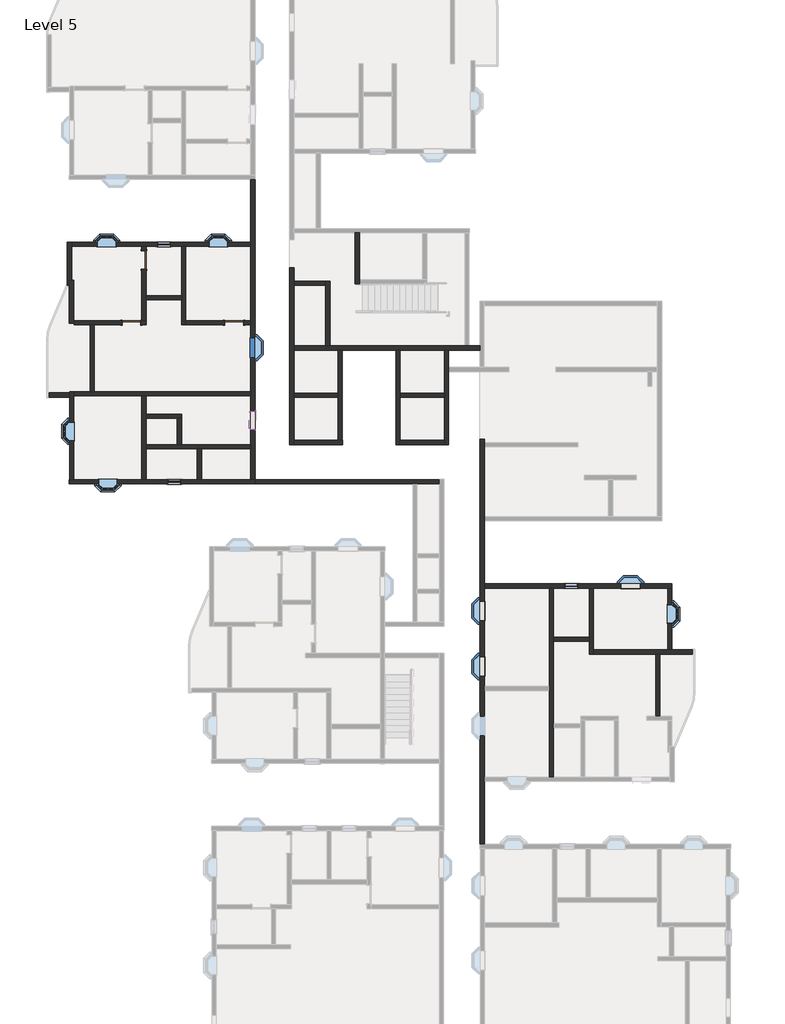
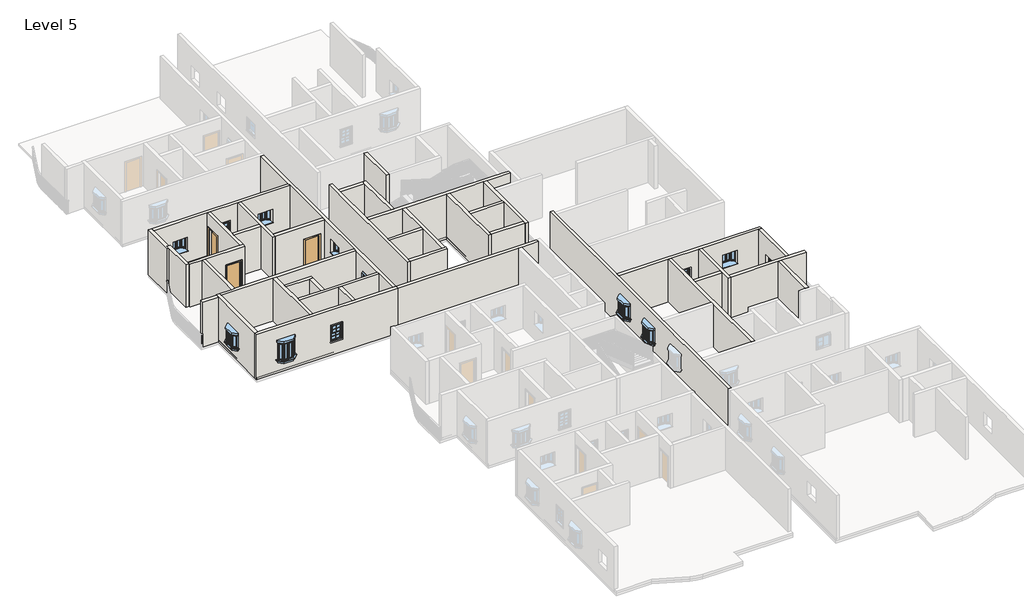
# One storey, part 3 of 14: 40 walls, 13 windows, 3 doors.
# Revit data of these elements (continued)
# Element 26 (IfcWall, "9\"")
#   Top Offset = 0' - 0"
#   Base Offset = 0' - 0"
#   wall height = 10' - 0"
#   Phase Created = New Construction
#   Base Constraint = Level 5
#   Top Constraint = Level 6
#   Materials on its faces: "Default Wall", "Earth"
# Element 27 (IfcWall, "9\"")
#   Top Offset = 0' - 0"
#   Base Offset = 0' - 0"
#   wall height = 10' - 0"
#   Phase Created = New Construction
#   Base Constraint = Level 5
#   Top Constraint = Level 6
#   Materials on its faces: "Default Wall", "Default Mass Interior Wall"
# Element 28 (IfcWall, "9\"")
#   Top Offset = 0' - 0"
#   Base Offset = 0' - 0"
#   wall height = 10' - 0"
#   Phase Created = New Construction
#   Base Constraint = Level 5
#   Top Constraint = Level 6
#   Materials on its faces: "Default Wall"
# Element 29 (IfcWall, "9\"")
#   Top Offset = 0' - 0"
#   Base Offset = 0' - 0"
#   wall height = 10' - 0"
#   Phase Created = New Construction
#   Base Constraint = Level 5
#   Top Constraint = Level 6
#   Materials on its faces: "Default Wall", "Default Mass Interior Wall", "Earth"
# Elements 30, 33, 34, 35, 36, 37, 38, 39, 40, 41 (IfcWall, "9\" w")
#   Top Offset = 0' - 0"
#   Base Offset = 0' - 0"
#   wall height = 10' - 0"
#   Phase Created = New Construction
#   Base Constraint = Level 5
#   Top Constraint = Level 6
#   Materials on its faces: "Default Wall"
# Element 31 (IfcWall, "9\" w")
#   Top Offset = 0' - 0"
#   Base Offset = 0' - 0"
#   wall height = 10' - 0"
#   Phase Created = New Construction
#   Base Constraint = Level 5
#   Top Constraint = Level 6
#   Materials on its faces: "Default Wall", "Earth"
# Element 32 (IfcWall, "9\" w")
#   Top Offset = 0' - 0"
#   Base Offset = 0' - 0"
#   wall height = 10' - 0"
#   Phase Created = New Construction
#   Base Constraint = Level 5
#   Top Constraint = Level 6
#   Materials on its faces: "Default Wall", "Brick, Soldier Course"
# Element 42 (IfcWall, "9\" w")
#   Top Offset = 0' - 0"
#   Base Offset = 0' - 0"
#   wall height = 10' - 0"
#   Phase Created = New Construction
#   Base Constraint = Level 5
#   Top Constraint = Level 6
#   Materials on its faces: "Default Wall", "Wood - Stained"
# Element 43 (IfcWall, "9\" w")
#   Top Offset = 0' - 0"
#   Base Offset = 0' - 0"
#   wall height = 10' - 0"
#   Phase Created = New Construction
#   Base Constraint = Level 5
#   Top Constraint = Level 6
#   Materials on its faces: "Default Wall", "Acoustic Ceiling Tile 24 x 24"
# Element 44 (IfcWindow, "910x1210mm")
#   Mark = "306"
#   Phase Created = New Construction
#   Materials on its faces: "Window Frame", "Glass"
# Element 45 (IfcWindow, "910x910mm")
#   Mark = "253"
#   Phase Created = New Construction
#   Materials on its faces: "Window Frame", "Glass"
# Element 46 (IfcWindow, "910x910mm")
#   Mark = "254"
#   Phase Created = New Construction
#   Materials on its faces: "Window Frame", "Glass"
# Element 47 (IfcWindow, "910x910mm")
#   Mark = "226"
#   Phase Created = New Construction
#   Materials on its faces: "Window Frame", "Glass"
# Element 48 (IfcWindow, "910x910mm")
#   Mark = "227"
#   Phase Created = New Construction
#   Materials on its faces: "Window Frame", "Glass"
# Element 49 (IfcWindow, "910x910mm")
#   Mark = "228"
#   Phase Created = New Construction
#   Materials on its faces: "Window Frame", "Glass"
# Element 50 (IfcWindow, "910x910mm")
#   Mark = "229"
#   Phase Created = New Construction
#   Materials on its faces: "Window Frame", "Glass"
# Element 51 (IfcWindow, "910x910mm")
#   Mark = "251"
#   Phase Created = New Construction
#   Materials on its faces: "Window Frame", "Glass"
# Element 52 (IfcWindow, "910x910mm")
#   Mark = "252"
#   Phase Created = New Construction
#   Materials on its faces: "Window Frame", "Glass"
# Element 53 (IfcWindow, "Window-Double-Hung : 26\" x 42\"")
#   Mark = "275"
#   Window Inset = 0' - 0"
#   Interior Wall Closure = 0' - 1 1/2"
#   Frame Extension = 0' - 1 1/4"
#   Exterior Wall Closure = 0' - 0 1/2"
#   Interior Trim Visibility = yes
#   Indicator Visibility = yes
#   Exterior Trim Visibility = yes
#   Phase Created = New Construction
#   Materials on its faces: "Wood - Stained", "Glass", "Clad - White"
# Element 54 (IfcWindow, "Window-Double-Hung : 26\" x 42\"")
#   Mark = "264"
#   Window Inset = 0' - 0"
#   Interior Wall Closure = 0' - 1 1/2"
#   Frame Extension = 0' - 1 1/4"
#   Exterior Wall Closure = 0' - 0 1/2"
#   Interior Trim Visibility = yes
#   Indicator Visibility = yes
#   Exterior Trim Visibility = yes
#   Phase Created = New Construction
#   Materials on its faces: "Wood - Stained", "Glass", "Clad - White"
# Element 55 (IfcWindow, "Window-Double-Hung : 26\" x 42\"")
#   Mark = "265"
#   Window Inset = 0' - 0"
#   Interior Wall Closure = 0' - 1 1/2"
#   Frame Extension = 0' - 1 1/4"
#   Exterior Wall Closure = 0' - 0 1/2"
#   Interior Trim Visibility = yes
#   Indicator Visibility = yes
#   Exterior Trim Visibility = yes
#   Phase Created = New Construction
#   Materials on its faces: "Wood - Stained", "Glass", "Clad - White"
# Element 56 (IfcWindow, "Windows_Sgl_w-Glazing_Bars : 910x910mm")
#   Mark = "260"
#   Phase Created = New Construction
#   Materials on its faces: "Window Frame", "Glass"
# Materials
#   "Door - Panel": class "Wood", colour RGB 210 159 95, transparency 0, Cost = 0
#   "Door - Frame": colour RGB 118 70 51, transparency 0, Cost = 0
#   "Window Frame": colour RGB 249 249 249, transparency 0
#   "Glass": class "Glass", colour RGB 0 128 192, transparency 0.75, Description = "Soda Lime Glass", Cost = 0
#   "Wood - Stained": class "Wood", colour RGB 224 178 126, transparency 0, Cost = 0
#   "Clad - White": class "Wood", colour RGB 242 242 238, transparency 0, Cost = 0
#   "Default Wall": colour RGB 128 128 128, transparency 0, Cost = 0
#   "Cherry": class "Wood", colour RGB 226 177 128, transparency 0, Description = "Prunus Serotina", Cost = 0
#   "Parking Stripe": class "Paint", colour RGB 250 250 91, transparency 0, Cost = 0
#   "Earth": class "Generic", colour RGB 97 75 62, transparency 0, Description = "Soil", Cost = 0
#   "Default Mass Interior Wall": class "Generic", colour RGB 195 229 126, transparency 0, Cost = 0
#   "Brick, Soldier Course": class "Masonry", colour RGB 170 98 104, transparency 0, Description = "Common brick soldier coursed", Cost = 0
#   "Acoustic Ceiling Tile 24 x 24": class "Generic", colour RGB 232 232 232, transparency 0, Description = "Acoustic Ceiling Tile 24 x 24", Cost = 0
